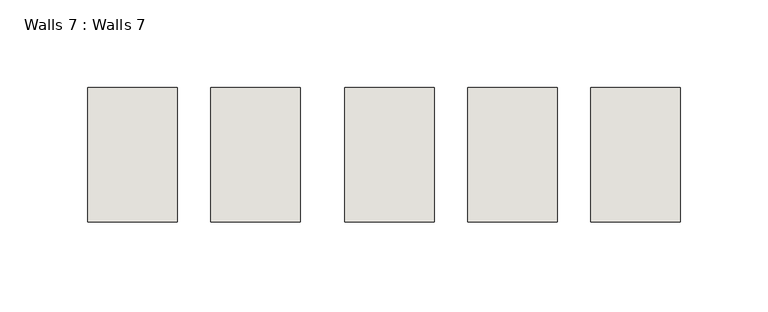
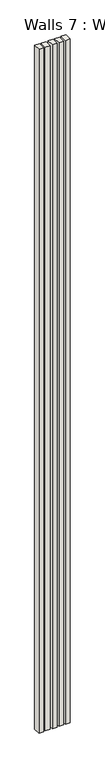
"""IFC4 building model written with IfcOpenShell, lengths in millimetres: wall geometry, Walls 7 : Walls 7."""

from ifc_helpers import new_model, si_unit, frame, origin, place, context, project, spatial, polyline, outline, extrude, source, transform, mapped, element, save


def walls_7_walls_7_9077e6f4(model_context):
    return source(origin(), model_context, "Body", "SweptSolid", [
        extrude(outline(polyline([(-3705.4569651, 155.2466379), (-3705.4569651, 79.0466379), (-3756.2569651, 79.0466379), (-3756.2569651, 155.2466379), (-3705.4569651, 155.2466379)])), frame((0.0, 0.0, 9144.0), z_axis=(0.0, 0.0, 1.0), x_axis=(1.0, 0.0, 0.0)), (0.0, 0.0, 1.0), 7770.9555037),
        extrude(outline(polyline([(-3775.3069651, 155.2466379), (-3775.3069651, 79.0466379), (-3826.1069651, 79.0466379), (-3826.1069651, 155.2466379), (-3775.3069651, 155.2466379)])), frame((0.0, 0.0, 9144.0), z_axis=(0.0, 0.0, 1.0), x_axis=(1.0, 0.0, 0.0)), (0.0, 0.0, 1.0), 7770.9555037),
        extrude(outline(polyline([(-3845.1569651, 155.2466379), (-3845.1569651, 79.0466379), (-3895.9569651, 79.0466379), (-3895.9569651, 155.2466379), (-3845.1569651, 155.2466379)])), frame((0.0, 0.0, 9144.0), z_axis=(0.0, 0.0, 1.0), x_axis=(1.0, 0.0, 0.0)), (0.0, 0.0, 1.0), 7770.9555037),
        extrude(outline(polyline([(-3921.3569651, 155.2466379), (-3921.3569651, 79.0466379), (-3972.1569651, 79.0466379), (-3972.1569651, 155.2466379), (-3921.3569651, 155.2466379)])), frame((0.0, 0.0, 9144.0), z_axis=(0.0, 0.0, 1.0), x_axis=(1.0, 0.0, 0.0)), (0.0, 0.0, 1.0), 7770.9555037),
        extrude(outline(polyline([(-3991.2069651, 155.2466379), (-3991.2069651, 79.0466379), (-4042.0069651, 79.0466379), (-4042.0069651, 155.2466379), (-3991.2069651, 155.2466379)])), frame((0.0, 0.0, 9144.0), z_axis=(0.0, 0.0, 1.0), x_axis=(1.0, 0.0, 0.0)), (0.0, 0.0, 1.0), 7770.9555037),
    ])


if __name__ == "__main__":
    model = new_model("IFC4")
    model_context = context("Model", 3, world=origin())
    ifc_project = project(units=[si_unit("LENGTHUNIT", "METRE", prefix="MILLI")], contexts=[model_context])
    site = spatial("IfcSite", under=ifc_project)
    building = spatial("IfcBuilding", under=site)
    placement = place(None, origin())
    walls_7_walls_7_shape = walls_7_walls_7_9077e6f4(model_context)
    element("IfcWall", 1, ObjectType="Walls 7 : Walls 7", at=placement, inside=building, context=model_context, shape_type="MappedRepresentation", body=[
        mapped(walls_7_walls_7_shape, transform((0.0, 0.0, 0.0), x_axis=(1.0, 0.0, 0.0), y_axis=(0.0, 1.0, 0.0), z_axis=(0.0, 0.0, 1.0))),
    ])
    save(model, "model.ifc")

# Revit data of these elements
# Element 1 (IfcWall, "Walls 7 : Walls 7")
#   Materials on its faces: "1 wood", "Default Wall"
# Materials
#   "1 wood": class "Generic", colour RGB 120 120 120, transparency 0, Cost = 0
#   "Default Wall": colour RGB 128 128 128, transparency 0, Cost = 0
